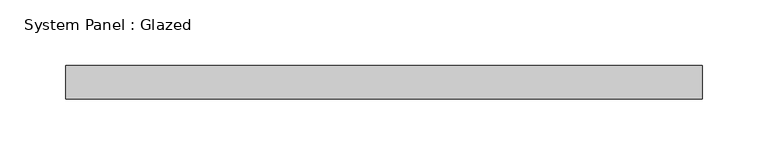
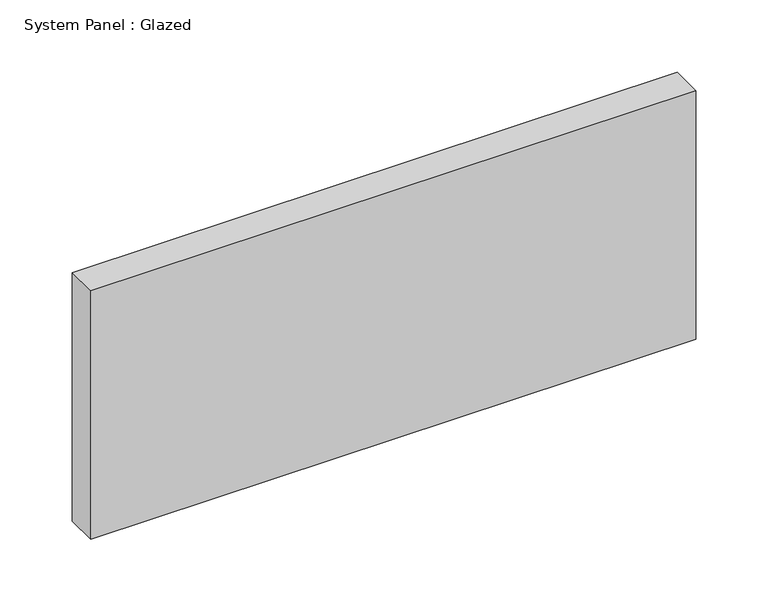
"""IFC4 building model written with IfcOpenShell, lengths in millimetres: plate geometry, System Panel : Glazed."""

from ifc_helpers import new_model, si_unit, origin, origin_with_axes, place, context, project, spatial, polyline, outline, extrude, source, transform, mapped, element, save


def system_panel_glazed_6bbf35ba(model_context):
    return source(origin(), model_context, "Body", "SweptSolid", [
        extrude(outline(polyline([(241.3, 19.05), (-241.3, 19.05), (-241.3, 44.45), (241.3, 44.45), (241.3, 19.05)])), origin_with_axes(), (0.0, 0.0, 1.0), 209.55),
    ])


if __name__ == "__main__":
    model = new_model("IFC4")
    model_context = context("Model", 3, world=origin())
    ifc_project = project(units=[si_unit("LENGTHUNIT", "METRE", prefix="MILLI")], contexts=[model_context])
    site = spatial("IfcSite", under=ifc_project)
    building = spatial("IfcBuilding", under=site)
    placement = place(None, origin())
    system_panel_glazed_shape = system_panel_glazed_6bbf35ba(model_context)
    element("IfcPlate", 1, ObjectType="System Panel : Glazed", at=placement, inside=building, context=model_context, shape_type="MappedRepresentation", body=[
        mapped(system_panel_glazed_shape, transform((0.0, 0.0, 0.0), x_axis=(1.0, 0.0, 0.0), y_axis=(0.0, 1.0, 0.0), z_axis=(0.0, 0.0, 1.0))),
    ])
    save(model, "model.ifc")

# Revit data of these elements
# Type "System Panel : Glazed"
#   Construction Type Id = "GSP4R"
#   Analytic Construction = "1/8 in Pilkington single glazing"
#   Visual Light Transmittance = 0.9
#   Solar Heat Gain Coefficient = 0.86
#   Heat Transfer Coefficient (U) = 1.18115 BTU/(h·ft²·°F)
#   Define Thermal Properties by = 1
# Element 1 (IfcPlate, "System Panel : Glazed")
#   Materials on its faces: "Glass"
# Materials
#   "Glass": class "Glass", colour RGB 0 128 192, transparency 0.75, Description = "Soda Lime Glass", Cost = 0
